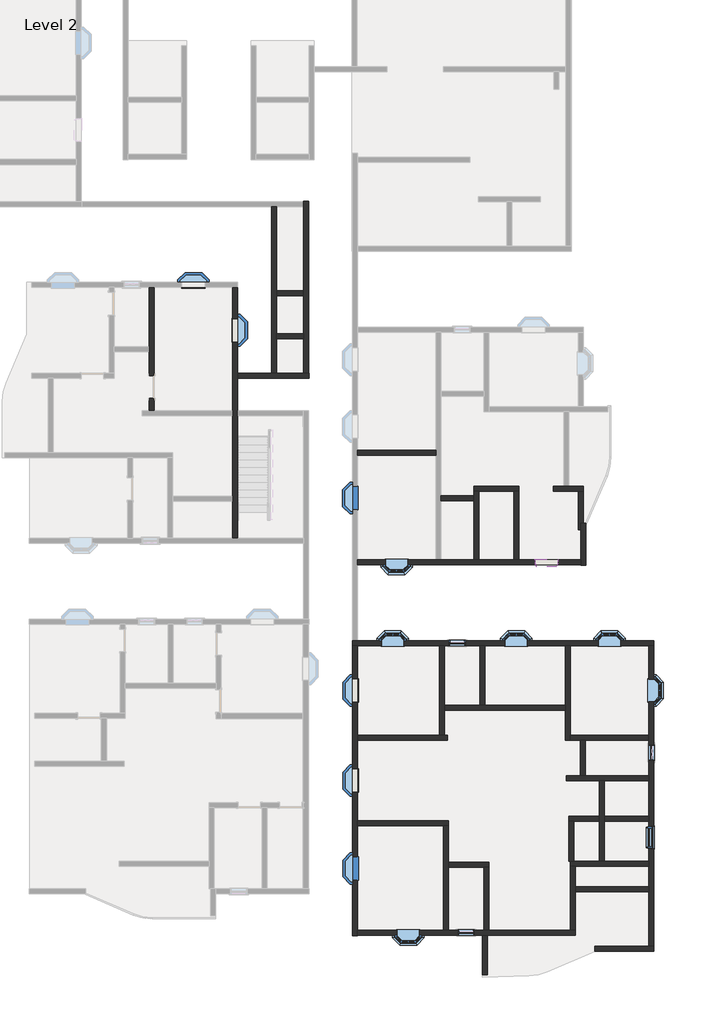
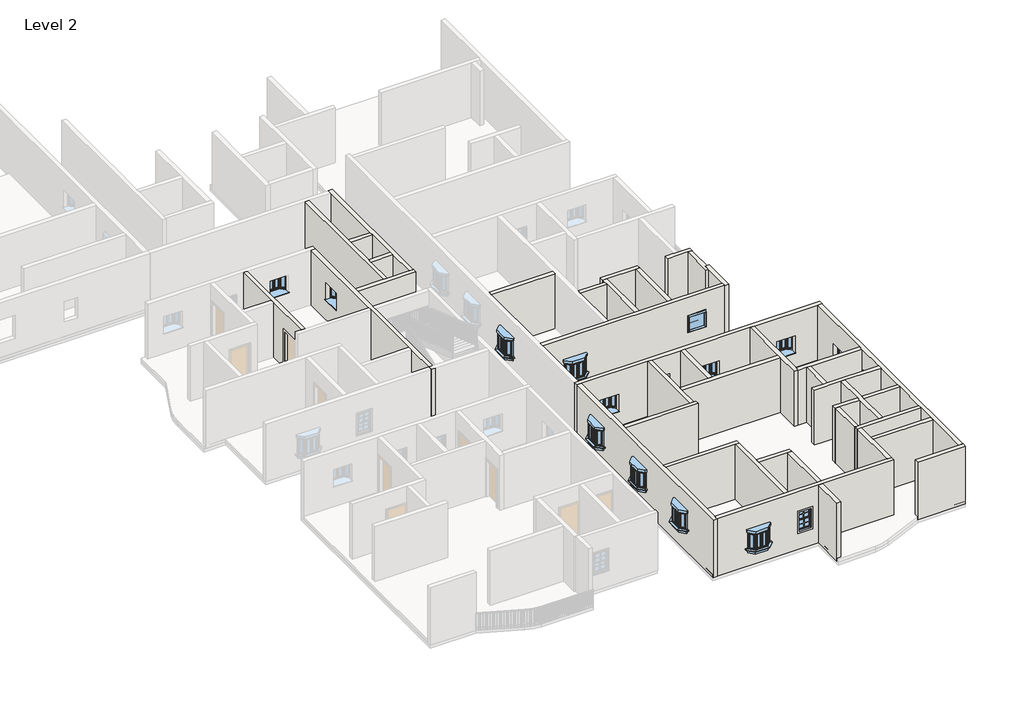
# One storey, part 2 of 14: 40 walls, 17 windows.
# Revit data of these elements (continued)
# Element 46 (IfcWindow, "910x910mm") (continued)
#   Phase Created = New Construction
#   Materials on its faces: "Window Frame", "Glass"
# Element 47 (IfcWindow, "910x910mm")
#   Mark = "82"
#   Phase Created = New Construction
#   Materials on its faces: "Window Frame", "Glass"
# Element 48 (IfcWindow, "910x910mm")
#   Mark = "83"
#   Phase Created = New Construction
#   Materials on its faces: "Window Frame", "Glass"
# Element 49 (IfcWindow, "910x910mm")
#   Mark = "84"
#   Phase Created = New Construction
#   Materials on its faces: "Window Frame", "Glass"
# Element 50 (IfcWindow, "910x910mm")
#   Mark = "85"
#   Phase Created = New Construction
#   Materials on its faces: "Window Frame", "Glass"
# Element 51 (IfcWindow, "910x910mm")
#   Mark = "86"
#   Phase Created = New Construction
#   Materials on its faces: "Window Frame", "Glass"
# Element 52 (IfcWindow, "910x910mm")
#   Mark = "87"
#   Phase Created = New Construction
#   Materials on its faces: "Window Frame", "Glass"
# Element 53 (IfcWindow, "Window-Double-Hung : 26\" x 42\"")
#   Mark = "110"
#   Window Inset = 0' - 0"
#   Interior Wall Closure = 0' - 1 1/2"
#   Frame Extension = 0' - 1 1/4"
#   Exterior Wall Closure = 0' - 0 1/2"
#   Interior Trim Visibility = yes
#   Indicator Visibility = yes
#   Exterior Trim Visibility = yes
#   Phase Created = New Construction
#   Materials on its faces: "Wood - Stained", "Glass", "Clad - White"
# Element 54 (IfcWindow, "Window-Double-Hung : 26\" x 42\"")
#   Mark = "111"
#   Window Inset = 0' - 0"
#   Interior Wall Closure = 0' - 1 1/2"
#   Frame Extension = 0' - 1 1/4"
#   Exterior Wall Closure = 0' - 0 1/2"
#   Interior Trim Visibility = yes
#   Indicator Visibility = yes
#   Exterior Trim Visibility = yes
#   Phase Created = New Construction
#   Materials on its faces: "Wood - Stained", "Glass", "Clad - White"
# Element 55 (IfcWindow, "Window-Double-Hung : 26\" x 42\"")
#   Mark = "112"
#   Window Inset = 0' - 0"
#   Interior Wall Closure = 0' - 1 1/2"
#   Frame Extension = 0' - 1 1/4"
#   Exterior Wall Closure = 0' - 0 1/2"
#   Interior Trim Visibility = yes
#   Indicator Visibility = yes
#   Exterior Trim Visibility = yes
#   Phase Created = New Construction
#   Materials on its faces: "Wood - Stained", "Glass", "Clad - White"
# Element 56 (IfcWindow, "Windows_Sgl_w-Glazing_Bars : 910x910mm")
#   Mark = "100"
#   Phase Created = New Construction
#   Materials on its faces: "Window Frame", "Glass"
# Element 57 (IfcWindow, "Windows_Sgl_w-Glazing_Bars : 910x910mm")
#   Mark = "99"
#   Phase Created = New Construction
#   Materials on its faces: "Window Frame", "Glass"
# Materials
#   "Window Frame": colour RGB 249 249 249, transparency 0
#   "Glass": class "Glass", colour RGB 0 128 192, transparency 0.75, Description = "Soda Lime Glass", Cost = 0
#   "Wood - Stained": class "Wood", colour RGB 224 178 126, transparency 0, Cost = 0
#   "Clad - White": class "Wood", colour RGB 242 242 238, transparency 0, Cost = 0
#   "Default Wall": colour RGB 128 128 128, transparency 0, Cost = 0
#   "Door - Frame": colour RGB 118 70 51, transparency 0, Cost = 0
#   "Earth": class "Generic", colour RGB 97 75 62, transparency 0, Description = "Soil", Cost = 0
#   "Carpet (1)": class "Carpet", colour RGB 124 80 67, transparency 0, Description = "Interior finish", Cost = 0
#   "Softwood, Lumber": class "Wood", colour RGB 223 192 134, transparency 0, Description = "Pinus Echinata", Cost = 0
#   "Acoustic Ceiling Tile 24 x 24": class "Generic", colour RGB 232 232 232, transparency 0, Description = "Acoustic Ceiling Tile 24 x 24", Cost = 0
